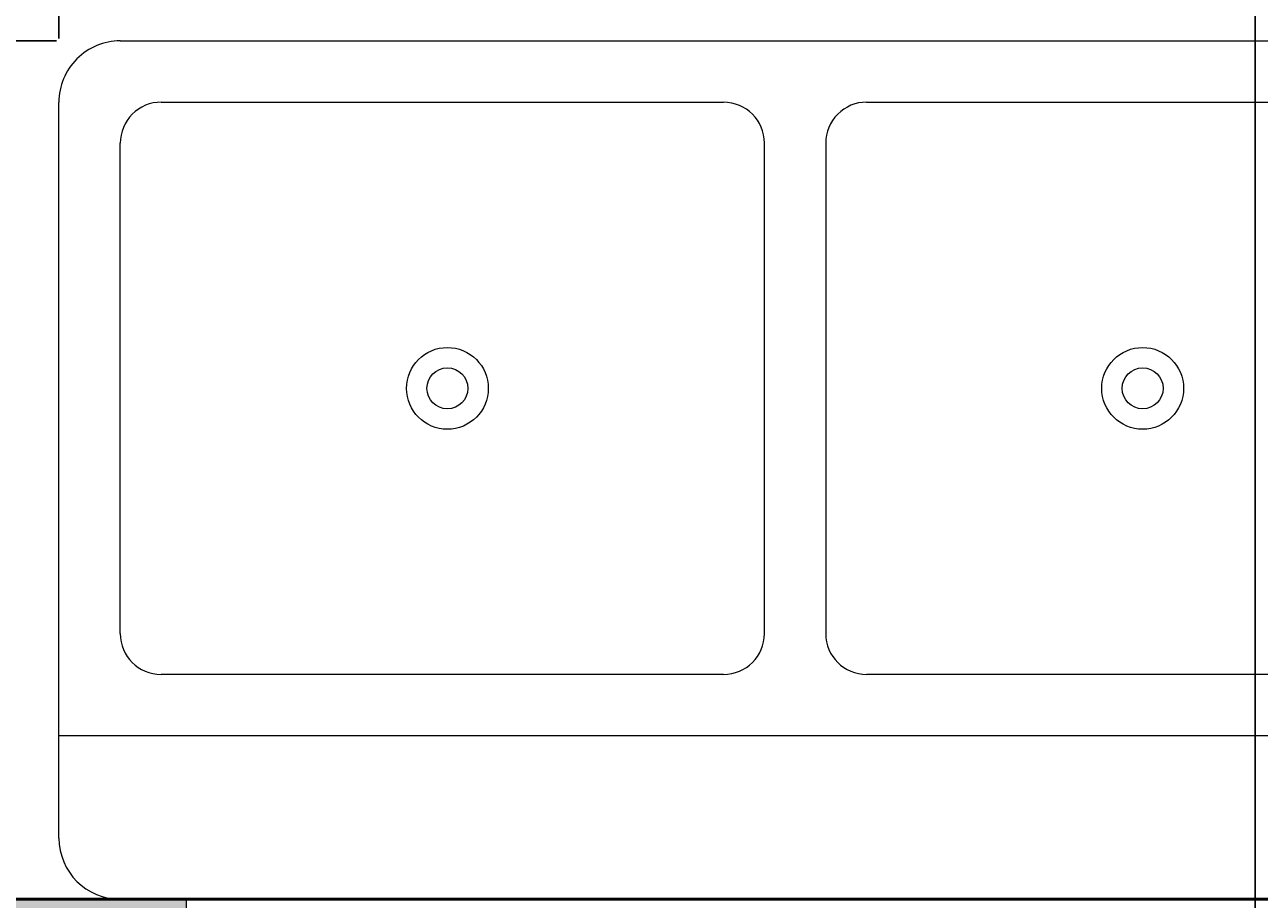
# Model space of a CAD drawing. Units: inches. Extents: x 2231 to 2461, y 2045 to 2455.
# Tile 19 of 95: x 2365 to 2395, y 2073 to 2094. Entities that reach past the tile are written whole.
import ezdxf

# ---------------------------------------------------------------- set-up
doc = ezdxf.new("R2010")
doc.units = ezdxf.units.IN
for name, color, linetype, lineweight in [('A-ANNO-DIMS', 2, 'Continuous', 18), ('A-FLOR-FIXT', 9, 'Continuous', 18), ('A-GLAZ', 4, 'Continuous', 18), ('A-WALL', 7, 'Continuous', 50)]:
    doc.layers.add(name, color=color, linetype=linetype, lineweight=lineweight)
doc.layers.add('A-WALL-PATT', color=18, linetype='Continuous', lineweight=13, true_color=0x000000)
doc.styles.get("Standard").update_dxf_attribs({"font": 'arial.ttf'})
doc.dimstyles.get("Standard").update_dxf_attribs({"dimtxt": 0.18, "dimasz": 0.18, "dimexe": 0.18, "dimexo": 0.0625, "dimgap": 0.09, "dimtad": 0, "dimtih": 1, "dimtoh": 1, "dimdec": 4, "dimzin": 0, "dimdsep": 46, "dimtxsty": 'Standard', "dimcen": 0.09, "dimadec": 0, "dimazin": 0, "dimtfac": 1, "dimtdec": 4, "dimtofl": 0, "dimtmove": 0, "dimatfit": 3, "dimfxl": 1, "dimtolj": 1, "dimtzin": 0, "dimarcsym": 0})

# ---------------------------------------------------------------- blocks, each defined once
blk = doc.blocks.new('Sink-double - 36 in top')
for p, q in [((-18, -4), (18, -4)), ((-0.75, -18.5), (-0.75, -6.5)), ((0.75, -6.5), (0.75, -18.5))]:
    blk.add_line(p, q)
for points in [[(-16.5, 0), (16.5, 0)], [(18, -1.5), (18, -19.5)], [(-15.5, -5.5), (-1.75, -5.5)], [(1.75, -5.5), (15.5, -5.5)], [(16.5, -6.5), (16.5, -18.5)], [(-1.75, -19.5), (-15.5, -19.5)], [(15.5, -19.5), (1.75, -19.5)], [(16.5, -21), (-16.5, -21)]]:
    blk.add_lwpolyline(points)
for centre, radius in [((-8.5, -12.5), 1), ((8.5, -12.5), 1), ((-8.5, -12.5), 0.5), ((8.5, -12.5), 0.5)]:
    blk.add_circle(centre, radius)
for centre, radius, start, end in [((16.5, -1.5), 1.5, 0, 90), ((-1.75, -6.5), 1, 0, 90), ((1.75, -6.5), 1, 90, 180), ((15.5, -6.5), 1, 0, 90), ((-1.75, -18.5), 1, 270, 0), ((1.75, -18.5), 1, 180, 270), ((15.5, -18.5), 1, 270, 0), ((16.5, -19.5), 1.5, 270, 0)]:
    blk.add_arc(centre, radius, start, end)
blk = doc.blocks.new('WIN-48IN')
blk.add_line((0, 0), (0, 9))
blk = doc.blocks.new('*D29')
at = {"layer": 'A-ANNO-DIMS', "color": 0, "lineweight": -2, "transparency": 16777216}
for p, q in [((2365.54, 2093.895), (2365.54, 2099.413)), ((2401.54, 2093.895), (2401.54, 2099.413)), ((2365.72, 2099.233), (2382.993, 2099.233)), ((2401.36, 2099.233), (2384.087, 2099.233))]:
    blk.add_line(p, q, dxfattribs=at)
at = {"layer": 'A-ANNO-DIMS', "color": 0, "transparency": 16777216}
for points in [[(2365.72, 2099.263), (2365.72, 2099.203), (2365.54, 2099.233)], [(2401.36, 2099.263), (2401.36, 2099.203), (2401.54, 2099.233)]]:
    blk.add_solid(points, dxfattribs=at)
at = {"layer": 'Defpoints', "color": 0, "transparency": 16777216}
for p in [(2365.54, 2099.233), (2365.54, 2093.833), (2401.54, 2093.833)]:
    blk.add_point(p, dxfattribs=at)
at = {"layer": 'A-ANNO-DIMS', "color": 0, "transparency": 16777216, "insert": (2383.54, 2099.233), "char_height": 0.18, "attachment_point": 5}
blk.add_mtext('\\A1;SINK 36', dxfattribs=at)
blk = doc.blocks.new('*D30')
at = {"layer": 'A-ANNO-DIMS', "color": 0, "lineweight": -2, "transparency": 16777216}
for p, q in [((2365.477, 2093.833), (2359.96, 2093.833)), ((2360.14, 2093.653), (2360.14, 2083.513)), ((2360.14, 2073.013), (2360.14, 2083.152)), ((2365.477, 2072.833), (2359.96, 2072.833))]:
    blk.add_line(p, q, dxfattribs=at)
at = {"layer": 'A-ANNO-DIMS', "color": 0, "transparency": 16777216}
for points in [[(2360.11, 2093.653), (2360.17, 2093.653), (2360.14, 2093.833)], [(2360.11, 2073.013), (2360.17, 2073.013), (2360.14, 2072.833)]]:
    blk.add_solid(points, dxfattribs=at)
at = {"layer": 'Defpoints', "color": 0, "transparency": 16777216}
for p in [(2365.54, 2093.833), (2360.14, 2072.833), (2365.54, 2072.833)]:
    blk.add_point(p, dxfattribs=at)
at = {"layer": 'A-ANNO-DIMS', "color": 0, "transparency": 16777216, "insert": (2360.14, 2083.333), "char_height": 0.18, "attachment_point": 5}
blk.add_mtext('\\A1;21', dxfattribs=at)
blk = doc.blocks.new('*D69')
at = {"layer": 'A-ANNO-DIMS', "color": 0, "lineweight": -2, "transparency": 16777216}
for p, q in [((2340.667, 2189.285), (2340.667, 2044.803)), ((2394.794, 2186.77), (2394.794, 2044.803)), ((2340.847, 2044.983), (2367.337, 2044.983)), ((2394.614, 2044.983), (2368.124, 2044.983))]:
    blk.add_line(p, q, dxfattribs=at)
at = {"layer": 'A-ANNO-DIMS', "color": 0, "transparency": 16777216}
for points in [[(2340.847, 2045.013), (2340.847, 2044.953), (2340.667, 2044.983)], [(2394.614, 2045.013), (2394.614, 2044.953), (2394.794, 2044.983)]]:
    blk.add_solid(points, dxfattribs=at)
at = {"layer": 'Defpoints', "color": 0, "transparency": 16777216}
for p in [(2340.667, 2189.348), (2394.794, 2186.833), (2394.794, 2044.983)]:
    blk.add_point(p, dxfattribs=at)
at = {"layer": 'A-ANNO-DIMS', "color": 0, "transparency": 16777216, "insert": (2367.73, 2044.983), "char_height": 0.18, "attachment_point": 5}
blk.add_mtext('\\A1;54.13', dxfattribs=at)

msp = doc.modelspace()

# ---------------------------------------------------------------- hatches: boundary and pattern name
at = {"layer": 'A-WALL-PATT'}
h = msp.add_hatch(color=256, dxfattribs=at)
h.dxf.hatch_style = 1
h.paths.add_polyline_path([(2441.7935, 2269.1535), (2432.7935, 2269.1535), (2432.7935, 2186.8328), (2396.7935, 2186.8328), (2396.7935, 2286.8328), (2394.7935, 2286.8328), (2394.7935, 2186.8328), (2334.7935, 2186.8328), (2334.7935, 2182.8328), (2432.7935, 2182.8328), (2432.7935, 2072.8328), (2416.6639, 2072.8328), (2416.6639, 2063.8328), (2441.7935, 2063.8328)])
h.paths.add_polyline_path([(2368.6639, 2072.8328), (2367.04, 2072.8328), (2330.7942, 2072.8328), (2330.7397, 2063.8328), (2368.6639, 2063.8328)])
h.paths.add_polyline_path([(2300.7392, 2068.3328), (2300.7392, 2072.8328), (2298.7935, 2072.8328), (2294.7935, 2072.8328), (2258.7935, 2072.8328), (2258.7935, 2120.8328), (2294.7935, 2120.8328), (2298.7935, 2120.8328), (2298.7935, 2128.8328), (2294.7935, 2128.8328), (2294.7935, 2124.8328), (2258.7935, 2124.8328), (2258.7935, 2182.8328), (2294.7935, 2182.8328), (2294.7935, 2174.8328), (2298.7935, 2174.8328), (2298.7935, 2182.8328), (2304.7935, 2182.8328), (2304.7935, 2186.8328), (2258.7935, 2186.8328), (2258.7935, 2221.999), (2249.7935, 2221.999), (2249.7935, 2063.8328), (2300.7392, 2063.8328)])
h.paths.add_polyline_path([(2391.9338, 2435.8328), (2333.82, 2435.8328), (2333.82, 2426.8328), (2368.7935, 2426.8328), (2368.7935, 2374.9508), (2368.7935, 2370.8328), (2372.3935, 2370.8328), (2372.7935, 2370.8328), (2372.7935, 2426.8328), (2391.9338, 2426.8328)])
h.paths.add_polyline_path([(2441.7935, 2435.8328), (2415.9338, 2435.8328), (2415.9338, 2426.8328), (2432.7935, 2426.8328), (2432.7935, 2334.8328), (2372.7935, 2334.8328), (2372.7935, 2346.8328), (2368.7935, 2346.8328), (2368.7935, 2306.8328), (2360.7935, 2306.8328), (2360.7935, 2302.8328), (2368.7935, 2302.8328), (2372.7935, 2302.8328), (2372.7935, 2330.8328), (2432.7935, 2330.8328), (2432.7935, 2317.1535), (2441.7935, 2317.1535)])
h.paths.add_polyline_path([(2285.82, 2435.8328), (2249.7935, 2435.8328), (2249.7935, 2269.999), (2258.7935, 2269.999), (2258.7935, 2302.8328), (2318.8168, 2302.8328), (2330.7935, 2302.8328), (2330.7935, 2306.8328), (2258.7935, 2306.8328), (2258.7935, 2426.8328), (2285.82, 2426.8328)])

# ---------------------------------------------------------------- linework, layer by layer
at = {"layer": 'A-WALL'}
msp.add_line((2432.7935, 2072.8328), (2330.7942, 2072.8328), dxfattribs=at)

# ---------------------------------------------------------------- block references
at = {"layer": 'A-FLOR-FIXT', "rotation": 180}
msp.add_blockref('Sink-double - 36 in top', (2383.54, 2072.8328), dxfattribs=at)
at = {"layer": 'A-GLAZ'}
msp.add_blockref('WIN-48IN', (2368.6639, 2063.833), dxfattribs=at)

# ---------------------------------------------------------------- dimensions: what is measured, and where the dimension line sits
at = {"layer": 'A-ANNO-DIMS'}
dim = msp.add_linear_dim(base=(2394.7935, 2044.9825), p1=(2340.6673, 2189.3477), p2=(2394.7935, 2186.8328), dimstyle='Standard', override={"dimdec": 2, "dimlfac": 1, "dimrnd": 0, "dimzin": 0, "dimdsep": 46, "dimlunit": 2}, dxfattribs=at)
dim.commit()
dim.dimension.update_dxf_attribs({"geometry": '*D69', "text_midpoint": (2367.7304, 2044.9825)})
dim = msp.add_linear_dim(base=(2365.54, 2099.2328), p1=(2401.54, 2093.8328), p2=(2365.54, 2093.8328), angle=180, text='SINK <>', dimstyle='Standard', override={"dimdec": 0, "dimlfac": 1, "dimrnd": 0, "dimzin": 0, "dimdsep": 46, "dimlunit": 2}, dxfattribs=at)
dim.commit()
dim.dimension.update_dxf_attribs({"geometry": '*D29', "text_midpoint": (2383.54, 2099.2328)})
dim = msp.add_linear_dim(base=(2360.14, 2072.8328), p1=(2365.54, 2093.8328), p2=(2365.54, 2072.8328), angle=270, dimstyle='Standard', override={"dimdec": 0, "dimlfac": 1, "dimrnd": 0, "dimzin": 0, "dimdsep": 46, "dimlunit": 2}, dxfattribs=at)
dim.commit()
dim.dimension.update_dxf_attribs({"geometry": '*D30', "text_midpoint": (2360.14, 2083.3328)})

doc.saveas('drawing.dxf')
